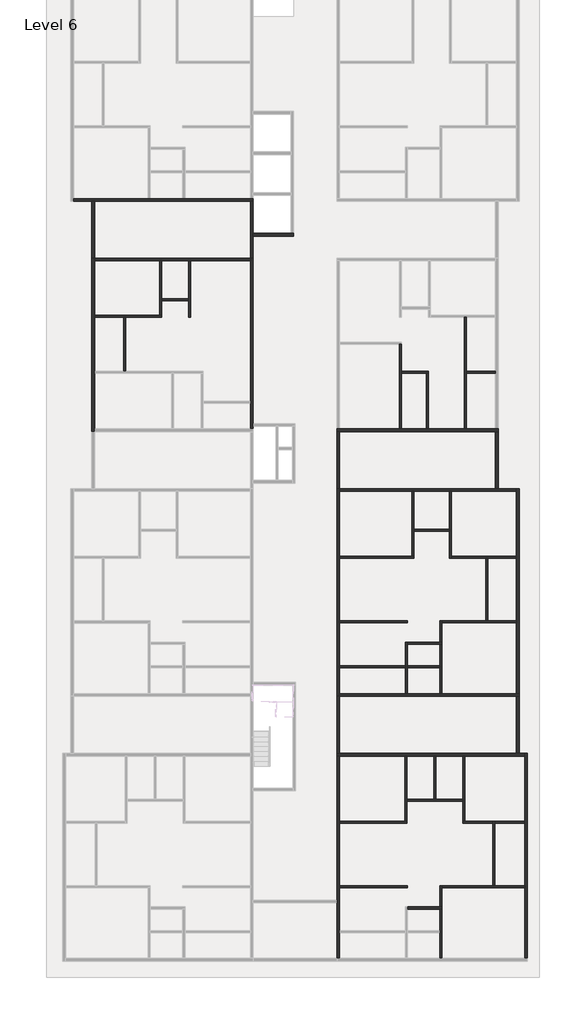
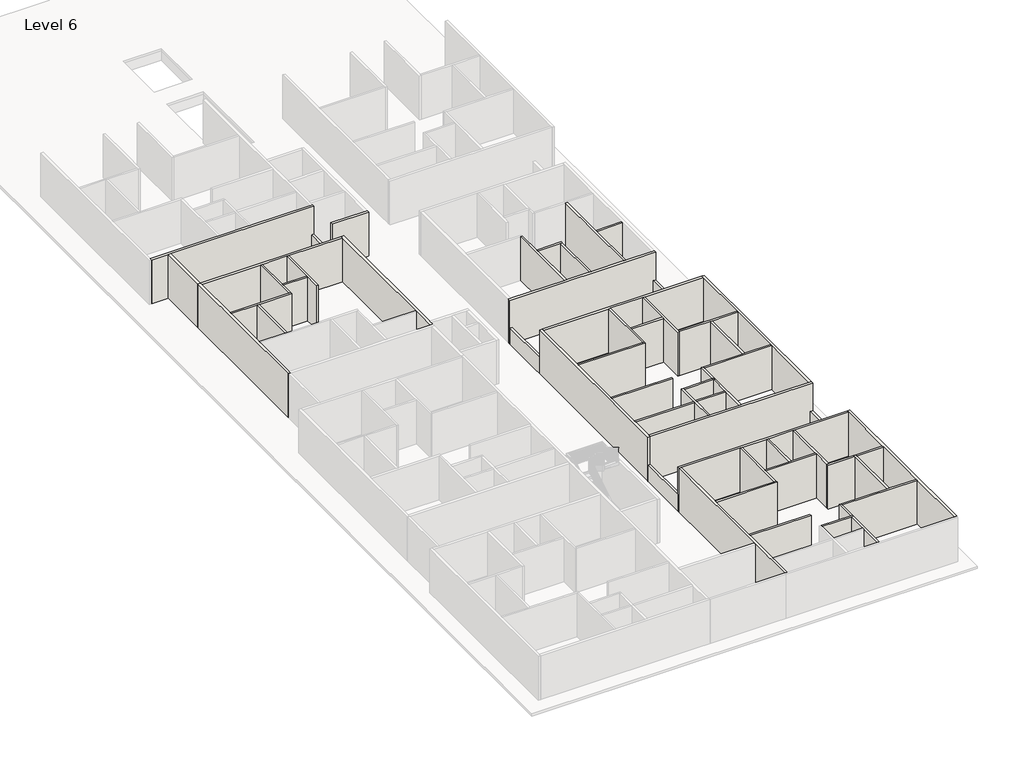
# One storey, part 2 of 8: 56 walls.
"""IFC4 building model written with IfcOpenShell, lengths in millimetres."""

from ifc_helpers import new_model, si_unit, frame, origin, place, context, project, spatial, polyline, outline, extrude, faceted_brep, element, save

model = new_model("IFC4")

# Units and contexts
model_context = context("Model", 3, world=origin())
ifc_project = project(units=[si_unit("LENGTHUNIT", "METRE", prefix="MILLI")], contexts=[model_context])

# Site, building, storey
site = spatial("IfcSite", under=ifc_project)
building = spatial("IfcBuilding", under=site)
storey = spatial("IfcBuildingStorey", under=building, Name="Level 6", Elevation=40474.6172466)

# Walls
placement = place(None, origin())
element("IfcWall", 1, ObjectType="4.5\"", at=placement, inside=storey, context=model_context, shape_type="Brep", body=[
    faceted_brep([(-12531.5544854, 2100.0216096, 40474.6172466), (-10907.2415084, 2100.0216096, 40474.6172466), (-10792.9415084, 2100.0216096, 40474.6172466), (-8759.6544854, 2100.0216096, 40474.6172466), (-8759.6544854, 2100.0216096, 43522.6172466), (-10792.9415084, 2100.0216096, 43522.6172466), (-10907.2415084, 2100.0216096, 43522.6172466), (-12531.5544854, 2100.0216096, 43522.6172466), (-12531.5544854, 2214.3216096, 40474.6172466), (-12531.5544854, 2214.3216096, 43522.6172466), (-8873.9544854, 2214.3216096, 43522.6172466), (-8759.6544854, 2214.3216096, 43522.6172466), (-8759.6544854, 2214.3216096, 40474.6172466), (-8873.9544854, 2214.3216096, 40474.6172466)], [[[0, 1, 2, 3, 4, 5, 6, 7]], [[8, 9, 10, 11, 12, 13]], [[3, 2, 1, 0, 8, 13, 12]], [[0, 7, 9, 8]], [[4, 3, 12, 11]], [[7, 6, 5, 4, 11, 10, 9]]]),
])
element("IfcWall", 2, ObjectType="4.5\"", at=placement, inside=storey, context=model_context, shape_type="Brep", body=[
    faceted_brep([(-8759.6544854, 2214.3216096, 40474.6172466), (-8759.6544854, 3014.4216096, 40474.6172466), (-8759.6544854, 3128.7216096, 40474.6172466), (-8759.6544854, 5264.2743917, 40474.6172466), (-8759.6544854, 5264.2743917, 43522.6172466), (-8759.6544854, 3128.7216096, 43522.6172466), (-8759.6544854, 3014.4216096, 43522.6172466), (-8759.6544854, 2214.3216096, 43522.6172466), (-8873.9544854, 2214.3216096, 40474.6172466), (-8873.9544854, 2214.3216096, 43522.6172466), (-8873.9544854, 5264.2743917, 43522.6172466), (-8873.9544854, 5264.2743917, 40474.6172466)], [[[0, 1, 2, 3, 4, 5, 6, 7]], [[8, 9, 10, 11]], [[3, 2, 1, 0, 8, 11]], [[0, 7, 9, 8]], [[4, 3, 11, 10]], [[7, 6, 5, 4, 10, 9]]]),
])
element("IfcWall", 3, ObjectType="4.5\"", at=placement, inside=storey, context=model_context, shape_type="Brep", body=[
    faceted_brep([(-7235.6544854, 5264.2743917, 40474.6172466), (-7235.6544854, 3128.7216096, 40474.6172466), (-7235.6544854, 3014.4216096, 40474.6172466), (-7235.6544854, 2100.0216096, 40474.6172466), (-7235.6544854, 2100.0216096, 43522.6172466), (-7235.6544854, 3014.4216096, 43522.6172466), (-7235.6544854, 3128.7216096, 43522.6172466), (-7235.6544854, 5264.2743917, 43522.6172466), (-7121.3544854, 5264.2743917, 40474.6172466), (-7121.3544854, 5264.2743917, 43522.6172466), (-7121.3544854, 2100.0216096, 43522.6172466), (-7121.3544854, 2100.0216096, 40474.6172466)], [[[0, 1, 2, 3, 4, 5, 6, 7]], [[8, 9, 10, 11]], [[3, 2, 1, 0, 8, 11]], [[4, 3, 11, 10]], [[0, 7, 9, 8]], [[7, 6, 5, 4, 10, 9]]]),
])
element("IfcWall", 4, ObjectType="4.5\"", at=placement, inside=storey, context=model_context, shape_type="SweptSolid", body=[
    extrude(outline(polyline([(-7235.6544854, 3014.4216096), (-8759.6544854, 3014.4216096), (-8759.6544854, 3128.7216096), (-7235.6544854, 3128.7216096), (-7235.6544854, 3014.4216096)])), frame((0.0, 0.0, 40474.6172466), z_axis=(0.0, 0.0, 1.0), x_axis=(1.0, 0.0, 0.0)), (0.0, 0.0, 1.0), 3048.0),
])
element("IfcWall", 5, ObjectType="4.5\"", at=placement, inside=storey, context=model_context, shape_type="SweptSolid", body=[
    extrude(outline(polyline([(-10907.2415084, -947.4344126), (-10907.2415084, 2100.0216096), (-10792.9415084, 2100.0216096), (-10792.9415084, -947.4344126), (-10907.2415084, -947.4344126)])), frame((0.0, 0.0, 40474.6172466), z_axis=(0.0, 0.0, 1.0), x_axis=(1.0, 0.0, 0.0)), (0.0, 0.0, 1.0), 3048.0),
])
element("IfcWall", 6, ObjectType="4.5\"", at=placement, inside=storey, context=model_context, shape_type="Brep", body=[
    faceted_brep([(5056.6584916, -31173.4344126, 40474.6172466), (6885.4584916, -31173.4344126, 40474.6172466), (6999.7584916, -31173.4344126, 40474.6172466), (6999.7584916, -31173.4344126, 43522.6172466), (6885.4584916, -31173.4344126, 43522.6172466), (5056.6584916, -31173.4344126, 43522.6172466), (5056.6584916, -31059.1344126, 40474.6172466), (5056.6584916, -31059.1344126, 43522.6172466), (6885.4584916, -31059.1344126, 43522.6172466), (6999.7584916, -31059.1344126, 43522.6172466), (6999.7584916, -31059.1344126, 40474.6172466), (6885.4584916, -31059.1344126, 40474.6172466)], [[[0, 1, 2, 3, 4, 5]], [[6, 7, 8, 9, 10, 11]], [[2, 1, 0, 6, 11, 10]], [[0, 5, 7, 6]], [[3, 2, 10, 9]], [[5, 4, 3, 9, 8, 7]]]),
])
element("IfcWall", 7, ObjectType="4.5\"", at=placement, inside=storey, context=model_context, shape_type="Brep", body=[
    faceted_brep([(6885.4584916, -31173.4344126, 40474.6172466), (6885.4584916, -32392.6344126, 40474.6172466), (6885.4584916, -32506.9344126, 40474.6172466), (6885.4584916, -33954.7344126, 40474.6172466), (6885.4584916, -33954.7344126, 43522.6172466), (6885.4584916, -32506.9344126, 43522.6172466), (6885.4584916, -32392.6344126, 43522.6172466), (6885.4584916, -31173.4344126, 43522.6172466), (6999.7584916, -31173.4344126, 40474.6172466), (6999.7584916, -31173.4344126, 43522.6172466), (6999.7584916, -33954.7344126, 43522.6172466), (6999.7584916, -33954.7344126, 40474.6172466)], [[[0, 1, 2, 3, 4, 5, 6, 7]], [[8, 9, 10, 11]], [[3, 2, 1, 0, 8, 11]], [[0, 7, 9, 8]], [[4, 3, 11, 10]], [[7, 6, 5, 4, 10, 9]]]),
])
element("IfcWall", 8, ObjectType="4.5\"", at=placement, inside=storey, context=model_context, shape_type="Brep", body=[
    faceted_brep([(6999.7584916, -31059.1344126, 40474.6172466), (6999.7584916, -29966.9344126, 40474.6172466), (6999.7584916, -29852.6344126, 40474.6172466), (6999.7584916, -29852.6344126, 43522.6172466), (6999.7584916, -29966.9344126, 43522.6172466), (6999.7584916, -31059.1344126, 43522.6172466), (6885.4584916, -31059.1344126, 40474.6172466), (6885.4584916, -31059.1344126, 43522.6172466), (6885.4584916, -29852.6344126, 43522.6172466), (6885.4584916, -29852.6344126, 40474.6172466)], [[[0, 1, 2, 3, 4, 5]], [[6, 7, 8, 9]], [[2, 1, 0, 6, 9]], [[0, 5, 7, 6]], [[3, 2, 9, 8]], [[5, 4, 3, 8, 7]]]),
])
element("IfcWall", 9, ObjectType="4.5\"", at=placement, inside=storey, context=model_context, shape_type="Brep", body=[
    faceted_brep([(6999.7584916, -29966.9344126, 40474.6172466), (11660.6584916, -29966.9344126, 40474.6172466), (11660.6584916, -29966.9344126, 43522.6172466), (6999.7584916, -29966.9344126, 43522.6172466), (6999.7584916, -29852.6344126, 40474.6172466), (6999.7584916, -29852.6344126, 43522.6172466), (9869.9584916, -29852.6344126, 43522.6172466), (9984.2584916, -29852.6344126, 43522.6172466), (11660.6584916, -29852.6344126, 43522.6172466), (11660.6584916, -29852.6344126, 40474.6172466), (9984.2584916, -29852.6344126, 40474.6172466), (9869.9584916, -29852.6344126, 40474.6172466)], [[[0, 1, 2, 3]], [[4, 5, 6, 7, 8, 9, 10, 11]], [[1, 0, 4, 11, 10, 9]], [[0, 3, 5, 4]], [[2, 1, 9, 8]], [[3, 2, 8, 7, 6, 5]]]),
])
element("IfcWall", 10, ObjectType="4.5\"", at=placement, inside=storey, context=model_context, shape_type="SweptSolid", body=[
    extrude(outline(polyline([(5056.6584916, -29966.9344126), (1259.3584916, -29966.9344126), (1259.3584916, -29852.6344126), (5056.6584916, -29852.6344126), (5056.6584916, -29966.9344126)])), frame((0.0, 0.0, 40474.6172466), z_axis=(0.0, 0.0, 1.0), x_axis=(1.0, 0.0, 0.0)), (0.0, 0.0, 1.0), 3048.0),
])
element("IfcWall", 11, ObjectType="4.5\"", at=placement, inside=storey, context=model_context, shape_type="Brep", body=[
    faceted_brep([(1259.3584916, -26347.4344126, 40474.6172466), (5031.2584916, -26347.4344126, 40474.6172466), (5031.2584916, -26347.4344126, 43522.6172466), (1259.3584916, -26347.4344126, 43522.6172466), (1259.3584916, -26233.1344126, 40474.6172466), (1259.3584916, -26233.1344126, 43522.6172466), (4916.9584916, -26233.1344126, 43522.6172466), (5031.2584916, -26233.1344126, 43522.6172466), (5031.2584916, -26233.1344126, 40474.6172466), (4916.9584916, -26233.1344126, 40474.6172466)], [[[0, 1, 2, 3]], [[4, 5, 6, 7, 8, 9]], [[1, 0, 4, 9, 8]], [[0, 3, 5, 4]], [[2, 1, 8, 7]], [[3, 2, 7, 6, 5]]]),
])
element("IfcWall", 12, ObjectType="4.5\"", at=placement, inside=storey, context=model_context, shape_type="Brep", body=[
    faceted_brep([(5031.2584916, -26233.1344126, 40474.6172466), (5031.2584916, -25128.2344126, 40474.6172466), (5031.2584916, -25013.9344126, 40474.6172466), (5031.2584916, -22575.5344126, 40474.6172466), (5031.2584916, -22575.5344126, 43522.6172466), (5031.2584916, -25013.9344126, 43522.6172466), (5031.2584916, -25128.2344126, 43522.6172466), (5031.2584916, -26233.1344126, 43522.6172466), (4916.9584916, -26233.1344126, 40474.6172466), (4916.9584916, -26233.1344126, 43522.6172466), (4916.9584916, -22575.5344126, 43522.6172466), (4916.9584916, -22575.5344126, 40474.6172466)], [[[0, 1, 2, 3, 4, 5, 6, 7]], [[8, 9, 10, 11]], [[3, 2, 1, 0, 8, 11]], [[0, 7, 9, 8]], [[4, 3, 11, 10]], [[7, 6, 5, 4, 10, 9]]]),
])
element("IfcWall", 13, ObjectType="4.5\"", at=placement, inside=storey, context=model_context, shape_type="Brep", body=[
    faceted_brep([(9984.2584916, -29852.6344126, 40474.6172466), (9984.2584916, -26347.4344126, 40474.6172466), (9984.2584916, -26233.1344126, 40474.6172466), (9984.2584916, -26233.1344126, 43522.6172466), (9984.2584916, -26347.4344126, 43522.6172466), (9984.2584916, -29852.6344126, 43522.6172466), (9869.9584916, -29852.6344126, 40474.6172466), (9869.9584916, -29852.6344126, 43522.6172466), (9869.9584916, -26347.4344126, 43522.6172466), (9869.9584916, -26233.1344126, 43522.6172466), (9869.9584916, -26233.1344126, 40474.6172466), (9869.9584916, -26347.4344126, 40474.6172466)], [[[0, 1, 2, 3, 4, 5]], [[6, 7, 8, 9, 10, 11]], [[2, 1, 0, 6, 11, 10]], [[0, 5, 7, 6]], [[3, 2, 10, 9]], [[5, 4, 3, 9, 8, 7]]]),
])
element("IfcWall", 14, ObjectType="4.5\"", at=placement, inside=storey, context=model_context, shape_type="SweptSolid", body=[
    extrude(outline(polyline([(11660.6584916, -26347.4344126), (9984.2584916, -26347.4344126), (9984.2584916, -26233.1344126), (11660.6584916, -26233.1344126), (11660.6584916, -26347.4344126)])), frame((0.0, 0.0, 40474.6172466), z_axis=(0.0, 0.0, 1.0), x_axis=(1.0, 0.0, 0.0)), (0.0, 0.0, 1.0), 3048.0),
])
element("IfcWall", 15, ObjectType="4.5\"", at=placement, inside=storey, context=model_context, shape_type="Brep", body=[
    faceted_brep([(9869.9584916, -26233.1344126, 40474.6172466), (8307.8584916, -26233.1344126, 40474.6172466), (8193.5584916, -26233.1344126, 40474.6172466), (8193.5584916, -26233.1344126, 43522.6172466), (8307.8584916, -26233.1344126, 43522.6172466), (9869.9584916, -26233.1344126, 43522.6172466), (9869.9584916, -26347.4344126, 40474.6172466), (9869.9584916, -26347.4344126, 43522.6172466), (8193.5584916, -26347.4344126, 43522.6172466), (8193.5584916, -26347.4344126, 40474.6172466)], [[[0, 1, 2, 3, 4, 5]], [[6, 7, 8, 9]], [[2, 1, 0, 6, 9]], [[0, 5, 7, 6]], [[3, 2, 9, 8]], [[5, 4, 3, 8, 7]]]),
])
element("IfcWall", 16, ObjectType="4.5\"", at=placement, inside=storey, context=model_context, shape_type="Brep", body=[
    faceted_brep([(8307.8584916, -26233.1344126, 40474.6172466), (8307.8584916, -22575.5344126, 40474.6172466), (8307.8584916, -22575.5344126, 43522.6172466), (8307.8584916, -26233.1344126, 43522.6172466), (8193.5584916, -26233.1344126, 40474.6172466), (8193.5584916, -26233.1344126, 43522.6172466), (8193.5584916, -25128.2344126, 43522.6172466), (8193.5584916, -25013.9344126, 43522.6172466), (8193.5584916, -22575.5344126, 43522.6172466), (8193.5584916, -22575.5344126, 40474.6172466), (8193.5584916, -25013.9344126, 40474.6172466), (8193.5584916, -25128.2344126, 40474.6172466)], [[[0, 1, 2, 3]], [[4, 5, 6, 7, 8, 9, 10, 11]], [[1, 0, 4, 11, 10, 9]], [[0, 3, 5, 4]], [[2, 1, 9, 8]], [[3, 2, 8, 7, 6, 5]]]),
])
element("IfcWall", 17, ObjectType="4.5\"", at=placement, inside=storey, context=model_context, shape_type="Brep", body=[
    faceted_brep([(5031.2584916, -25128.2344126, 40474.6172466), (8193.5584916, -25128.2344126, 40474.6172466), (8193.5584916, -25128.2344126, 43522.6172466), (5031.2584916, -25128.2344126, 43522.6172466), (5031.2584916, -25013.9344126, 40474.6172466), (5031.2584916, -25013.9344126, 43522.6172466), (6555.2584916, -25013.9344126, 43522.6172466), (6669.5584916, -25013.9344126, 43522.6172466), (8193.5584916, -25013.9344126, 43522.6172466), (8193.5584916, -25013.9344126, 40474.6172466), (6669.5584916, -25013.9344126, 40474.6172466), (6555.2584916, -25013.9344126, 40474.6172466)], [[[0, 1, 2, 3]], [[4, 5, 6, 7, 8, 9, 10, 11]], [[1, 0, 4, 11, 10, 9]], [[0, 3, 5, 4]], [[2, 1, 9, 8]], [[3, 2, 8, 7, 6, 5]]]),
])
element("IfcWall", 18, ObjectType="4.5\"", at=placement, inside=storey, context=model_context, shape_type="SweptSolid", body=[
    extrude(outline(polyline([(6555.2584916, -25013.9344126), (6555.2584916, -22575.5344126), (6669.5584916, -22575.5344126), (6669.5584916, -25013.9344126), (6555.2584916, -25013.9344126)])), frame((0.0, 0.0, 40474.6172466), z_axis=(0.0, 0.0, 1.0), x_axis=(1.0, 0.0, 0.0)), (0.0, 0.0, 1.0), 3048.0),
])
element("IfcWall", 19, ObjectType="4.5\"", at=placement, inside=storey, context=model_context, shape_type="SweptSolid", body=[
    extrude(outline(polyline([(4942.3584916, -17622.5344126), (1259.3584916, -17622.5344126), (1259.3584916, -17508.2344126), (4942.3584916, -17508.2344126), (4942.3584916, -17622.5344126)])), frame((0.0, 0.0, 40474.6172466), z_axis=(0.0, 0.0, 1.0), x_axis=(1.0, 0.0, 0.0)), (0.0, 0.0, 1.0), 3048.0),
])
element("IfcWall", 20, ObjectType="4.5\"", at=placement, inside=storey, context=model_context, shape_type="Brep", body=[
    faceted_brep([(4942.3584916, -16174.7344126, 40474.6172466), (4942.3584916, -17508.2344126, 40474.6172466), (4942.3584916, -17622.5344126, 40474.6172466), (4942.3584916, -19070.3344126, 40474.6172466), (4942.3584916, -19070.3344126, 43522.6172466), (4942.3584916, -17622.5344126, 43522.6172466), (4942.3584916, -17508.2344126, 43522.6172466), (4942.3584916, -16174.7344126, 43522.6172466), (5056.6584916, -16174.7344126, 40474.6172466), (5056.6584916, -16174.7344126, 43522.6172466), (5056.6584916, -16289.0344126, 43522.6172466), (5056.6584916, -17508.2344126, 43522.6172466), (5056.6584916, -17622.5344126, 43522.6172466), (5056.6584916, -19070.3344126, 43522.6172466), (5056.6584916, -19070.3344126, 40474.6172466), (5056.6584916, -17622.5344126, 40474.6172466), (5056.6584916, -17508.2344126, 40474.6172466), (5056.6584916, -16289.0344126, 40474.6172466)], [[[0, 1, 2, 3, 4, 5, 6, 7]], [[8, 9, 10, 11, 12, 13, 14, 15, 16, 17]], [[3, 2, 1, 0, 8, 17, 16, 15, 14]], [[4, 3, 14, 13]], [[0, 7, 9, 8]], [[7, 6, 5, 4, 13, 12, 11, 10, 9]]]),
])
element("IfcWall", 21, ObjectType="4.5\"", at=placement, inside=storey, context=model_context, shape_type="Brep", body=[
    faceted_brep([(5056.6584916, -16289.0344126, 40474.6172466), (6885.4584916, -16289.0344126, 40474.6172466), (6999.7584916, -16289.0344126, 40474.6172466), (6999.7584916, -16289.0344126, 43522.6172466), (6885.4584916, -16289.0344126, 43522.6172466), (5056.6584916, -16289.0344126, 43522.6172466), (5056.6584916, -16174.7344126, 40474.6172466), (5056.6584916, -16174.7344126, 43522.6172466), (6885.4584916, -16174.7344126, 43522.6172466), (6999.7584916, -16174.7344126, 43522.6172466), (6999.7584916, -16174.7344126, 40474.6172466), (6885.4584916, -16174.7344126, 40474.6172466)], [[[0, 1, 2, 3, 4, 5]], [[6, 7, 8, 9, 10, 11]], [[2, 1, 0, 6, 11, 10]], [[0, 5, 7, 6]], [[3, 2, 10, 9]], [[5, 4, 3, 9, 8, 7]]]),
])
element("IfcWall", 22, ObjectType="4.5\"", at=placement, inside=storey, context=model_context, shape_type="Brep", body=[
    faceted_brep([(6885.4584916, -16289.0344126, 40474.6172466), (6885.4584916, -17508.2344126, 40474.6172466), (6885.4584916, -17622.5344126, 40474.6172466), (6885.4584916, -19070.3344126, 40474.6172466), (6885.4584916, -19070.3344126, 43522.6172466), (6885.4584916, -17622.5344126, 43522.6172466), (6885.4584916, -17508.2344126, 43522.6172466), (6885.4584916, -16289.0344126, 43522.6172466), (6999.7584916, -16289.0344126, 40474.6172466), (6999.7584916, -16289.0344126, 43522.6172466), (6999.7584916, -19070.3344126, 43522.6172466), (6999.7584916, -19070.3344126, 40474.6172466)], [[[0, 1, 2, 3, 4, 5, 6, 7]], [[8, 9, 10, 11]], [[3, 2, 1, 0, 8, 11]], [[0, 7, 9, 8]], [[4, 3, 11, 10]], [[7, 6, 5, 4, 10, 9]]]),
])
element("IfcWall", 23, ObjectType="4.5\"", at=placement, inside=storey, context=model_context, shape_type="SweptSolid", body=[
    extrude(outline(polyline([(6885.4584916, -17622.5344126), (5056.6584916, -17622.5344126), (5056.6584916, -17508.2344126), (6885.4584916, -17508.2344126), (6885.4584916, -17622.5344126)])), frame((0.0, 0.0, 40474.6172466), z_axis=(0.0, 0.0, 1.0), x_axis=(1.0, 0.0, 0.0)), (0.0, 0.0, 1.0), 3048.0),
])
element("IfcWall", 24, ObjectType="4.5\"", at=placement, inside=storey, context=model_context, shape_type="Brep", body=[
    faceted_brep([(6999.7584916, -16174.7344126, 40474.6172466), (6999.7584916, -15082.5344126, 40474.6172466), (6999.7584916, -14968.2344126, 40474.6172466), (6999.7584916, -14968.2344126, 43522.6172466), (6999.7584916, -15082.5344126, 43522.6172466), (6999.7584916, -16174.7344126, 43522.6172466), (6885.4584916, -16174.7344126, 40474.6172466), (6885.4584916, -16174.7344126, 43522.6172466), (6885.4584916, -14968.2344126, 43522.6172466), (6885.4584916, -14968.2344126, 40474.6172466)], [[[0, 1, 2, 3, 4, 5]], [[6, 7, 8, 9]], [[2, 1, 0, 6, 9]], [[0, 5, 7, 6]], [[3, 2, 9, 8]], [[5, 4, 3, 8, 7]]]),
])
element("IfcWall", 25, ObjectType="4.5\"", at=placement, inside=storey, context=model_context, shape_type="Brep", body=[
    faceted_brep([(6999.7584916, -15082.5344126, 40474.6172466), (11208.5214687, -15082.5344126, 40474.6172466), (11208.5214687, -15082.5344126, 43522.6172466), (6999.7584916, -15082.5344126, 43522.6172466), (6999.7584916, -14968.2344126, 40474.6172466), (6999.7584916, -14968.2344126, 43522.6172466), (9469.9084916, -14968.2344126, 43522.6172466), (9584.2084916, -14968.2344126, 43522.6172466), (11208.5214687, -14968.2344126, 43522.6172466), (11208.5214687, -14968.2344126, 40474.6172466), (9584.2084916, -14968.2344126, 40474.6172466), (9469.9084916, -14968.2344126, 40474.6172466)], [[[0, 1, 2, 3]], [[4, 5, 6, 7, 8, 9, 10, 11]], [[1, 0, 4, 11, 10, 9]], [[0, 3, 5, 4]], [[2, 1, 9, 8]], [[3, 2, 8, 7, 6, 5]]]),
])
element("IfcWall", 26, ObjectType="4.5\"", at=placement, inside=storey, context=model_context, shape_type="SweptSolid", body=[
    extrude(outline(polyline([(5056.6584916, -15082.5344126), (1259.3584916, -15082.5344126), (1259.3584916, -14968.2344126), (5056.6584916, -14968.2344126), (5056.6584916, -15082.5344126)])), frame((0.0, 0.0, 40474.6172466), z_axis=(0.0, 0.0, 1.0), x_axis=(1.0, 0.0, 0.0)), (0.0, 0.0, 1.0), 3048.0),
])
element("IfcWall", 27, ObjectType="4.5\"", at=placement, inside=storey, context=model_context, shape_type="Brep", body=[
    faceted_brep([(1259.3584916, -11463.0344126, 40474.6172466), (5430.0214687, -11463.0344126, 40474.6172466), (5430.0214687, -11463.0344126, 43522.6172466), (1259.3584916, -11463.0344126, 43522.6172466), (1259.3584916, -11348.7344126, 40474.6172466), (1259.3584916, -11348.7344126, 43522.6172466), (5315.7214687, -11348.7344126, 43522.6172466), (5430.0214687, -11348.7344126, 43522.6172466), (5430.0214687, -11348.7344126, 40474.6172466), (5315.7214687, -11348.7344126, 40474.6172466)], [[[0, 1, 2, 3]], [[4, 5, 6, 7, 8, 9]], [[1, 0, 4, 9, 8]], [[0, 3, 5, 4]], [[2, 1, 8, 7]], [[3, 2, 7, 6, 5]]]),
])
element("IfcWall", 28, ObjectType="4.5\"", at=placement, inside=storey, context=model_context, shape_type="Brep", body=[
    faceted_brep([(5430.0214687, -11348.7344126, 40474.6172466), (5430.0214687, -9939.0344126, 40474.6172466), (5430.0214687, -9824.7344126, 40474.6172466), (5430.0214687, -7691.1344126, 40474.6172466), (5430.0214687, -7691.1344126, 43522.6172466), (5430.0214687, -9824.7344126, 43522.6172466), (5430.0214687, -9939.0344126, 43522.6172466), (5430.0214687, -11348.7344126, 43522.6172466), (5315.7214687, -11348.7344126, 40474.6172466), (5315.7214687, -11348.7344126, 43522.6172466), (5315.7214687, -7691.1344126, 43522.6172466), (5315.7214687, -7691.1344126, 40474.6172466)], [[[0, 1, 2, 3, 4, 5, 6, 7]], [[8, 9, 10, 11]], [[3, 2, 1, 0, 8, 11]], [[0, 7, 9, 8]], [[4, 3, 11, 10]], [[7, 6, 5, 4, 10, 9]]]),
])
element("IfcWall", 29, ObjectType="4.5\"", at=placement, inside=storey, context=model_context, shape_type="SweptSolid", body=[
    extrude(outline(polyline([(7436.6214687, -9939.0344126), (5430.0214687, -9939.0344126), (5430.0214687, -9824.7344126), (7436.6214687, -9824.7344126), (7436.6214687, -9939.0344126)])), frame((0.0, 0.0, 40474.6172466), z_axis=(0.0, 0.0, 1.0), x_axis=(1.0, 0.0, 0.0)), (0.0, 0.0, 1.0), 3048.0),
])
element("IfcWall", 30, ObjectType="4.5\"", at=placement, inside=storey, context=model_context, shape_type="Brep", body=[
    faceted_brep([(7436.6214687, -7691.1344126, 40474.6172466), (7436.6214687, -9824.7344126, 40474.6172466), (7436.6214687, -9939.0344126, 40474.6172466), (7436.6214687, -11463.0344126, 40474.6172466), (7436.6214687, -11463.0344126, 43522.6172466), (7436.6214687, -9939.0344126, 43522.6172466), (7436.6214687, -9824.7344126, 43522.6172466), (7436.6214687, -7691.1344126, 43522.6172466), (7550.9214687, -7691.1344126, 40474.6172466), (7550.9214687, -7691.1344126, 43522.6172466), (7550.9214687, -11348.7344126, 43522.6172466), (7550.9214687, -11463.0344126, 43522.6172466), (7550.9214687, -11463.0344126, 40474.6172466), (7550.9214687, -11348.7344126, 40474.6172466)], [[[0, 1, 2, 3, 4, 5, 6, 7]], [[8, 9, 10, 11, 12, 13]], [[3, 2, 1, 0, 8, 13, 12]], [[0, 7, 9, 8]], [[4, 3, 12, 11]], [[7, 6, 5, 4, 11, 10, 9]]]),
])
element("IfcWall", 31, ObjectType="4.5\"", at=placement, inside=storey, context=model_context, shape_type="Brep", body=[
    faceted_brep([(7550.9214687, -11463.0344126, 40474.6172466), (9469.9084916, -11463.0344126, 40474.6172466), (9584.2084916, -11463.0344126, 40474.6172466), (11208.5214687, -11463.0344126, 40474.6172466), (11208.5214687, -11463.0344126, 43522.6172466), (9584.2084916, -11463.0344126, 43522.6172466), (9469.9084916, -11463.0344126, 43522.6172466), (7550.9214687, -11463.0344126, 43522.6172466), (7550.9214687, -11348.7344126, 40474.6172466), (7550.9214687, -11348.7344126, 43522.6172466), (11208.5214687, -11348.7344126, 43522.6172466), (11208.5214687, -11348.7344126, 40474.6172466)], [[[0, 1, 2, 3, 4, 5, 6, 7]], [[8, 9, 10, 11]], [[3, 2, 1, 0, 8, 11]], [[0, 7, 9, 8]], [[4, 3, 11, 10]], [[7, 6, 5, 4, 10, 9]]]),
])
element("IfcWall", 32, ObjectType="4.5\"", at=placement, inside=storey, context=model_context, shape_type="SweptSolid", body=[
    extrude(outline(polyline([(9469.9084916, -14968.2344126), (9469.9084916, -11463.0344126), (9584.2084916, -11463.0344126), (9584.2084916, -14968.2344126), (9469.9084916, -14968.2344126)])), frame((0.0, 0.0, 40474.6172466), z_axis=(0.0, 0.0, 1.0), x_axis=(1.0, 0.0, 0.0)), (0.0, 0.0, 1.0), 3048.0),
])
element("IfcWall", 33, ObjectType="4.5\"", at=placement, inside=storey, context=model_context, shape_type="Brep", body=[
    faceted_brep([(4610.8714687, 572.7745083, 40474.6172466), (4610.8714687, -4185.9344126, 40474.6172466), (4610.8714687, -4185.9344126, 43522.6172466), (4610.8714687, 572.7745083, 43522.6172466), (4725.1714687, 572.7745083, 40474.6172466), (4725.1714687, 572.7745083, 43522.6172466), (4725.1714687, -947.4344126, 43522.6172466), (4725.1714687, -1061.7344126, 43522.6172466), (4725.1714687, -4185.9344126, 43522.6172466), (4725.1714687, -4185.9344126, 40474.6172466), (4725.1714687, -1061.7344126, 40474.6172466), (4725.1714687, -947.4344126, 40474.6172466)], [[[0, 1, 2, 3]], [[4, 5, 6, 7, 8, 9, 10, 11]], [[1, 0, 4, 11, 10, 9]], [[0, 3, 5, 4]], [[2, 1, 9, 8]], [[3, 2, 8, 7, 6, 5]]]),
])
element("IfcWall", 34, ObjectType="4.5\"", at=placement, inside=storey, context=model_context, shape_type="Brep", body=[
    faceted_brep([(4725.1714687, -1061.7344126, 40474.6172466), (6134.8714687, -1061.7344126, 40474.6172466), (6249.1714687, -1061.7344126, 40474.6172466), (6249.1714687, -1061.7344126, 43522.6172466), (6134.8714687, -1061.7344126, 43522.6172466), (4725.1714687, -1061.7344126, 43522.6172466), (4725.1714687, -947.4344126, 40474.6172466), (4725.1714687, -947.4344126, 43522.6172466), (6249.1714687, -947.4344126, 43522.6172466), (6249.1714687, -947.4344126, 40474.6172466)], [[[0, 1, 2, 3, 4, 5]], [[6, 7, 8, 9]], [[2, 1, 0, 6, 9]], [[0, 5, 7, 6]], [[3, 2, 9, 8]], [[5, 4, 3, 8, 7]]]),
])
element("IfcWall", 35, ObjectType="4.5\"", at=placement, inside=storey, context=model_context, shape_type="SweptSolid", body=[
    extrude(outline(polyline([(6134.8714687, -4185.9344126), (6134.8714687, -1061.7344126), (6249.1714687, -1061.7344126), (6249.1714687, -4185.9344126), (6134.8714687, -4185.9344126)])), frame((0.0, 0.0, 40474.6172466), z_axis=(0.0, 0.0, 1.0), x_axis=(1.0, 0.0, 0.0)), (0.0, 0.0, 1.0), 3048.0),
])
element("IfcWall", 36, ObjectType="4.5\"", at=placement, inside=storey, context=model_context, shape_type="Brep", body=[
    faceted_brep([(8396.7584916, -4185.9344126, 40474.6172466), (8396.7584916, -1061.7344126, 40474.6172466), (8396.7584916, -947.4344126, 40474.6172466), (8396.7584916, 2100.0216096, 40474.6172466), (8396.7584916, 2100.0216096, 43522.6172466), (8396.7584916, -947.4344126, 43522.6172466), (8396.7584916, -1061.7344126, 43522.6172466), (8396.7584916, -4185.9344126, 43522.6172466), (8282.4584916, -4185.9344126, 40474.6172466), (8282.4584916, -4185.9344126, 43522.6172466), (8282.4584916, 2100.0216096, 43522.6172466), (8282.4584916, 2100.0216096, 40474.6172466)], [[[0, 1, 2, 3, 4, 5, 6, 7]], [[8, 9, 10, 11]], [[3, 2, 1, 0, 8, 11]], [[0, 7, 9, 8]], [[4, 3, 11, 10]], [[7, 6, 5, 4, 10, 9]]]),
])
element("IfcWall", 37, ObjectType="4.5\"", at=placement, inside=storey, context=model_context, shape_type="SweptSolid", body=[
    extrude(outline(polyline([(8396.7584916, -947.4344126), (10021.0714687, -947.4344126), (10021.0714687, -1061.7344126), (8396.7584916, -1061.7344126), (8396.7584916, -947.4344126)])), frame((0.0, 0.0, 40474.6172466), z_axis=(0.0, 0.0, 1.0), x_axis=(1.0, 0.0, 0.0)), (0.0, 0.0, 1.0), 3048.0),
])
element("IfcWall", 38, ObjectType="6\"", at=placement, inside=storey, context=model_context, shape_type="Brep", body=[
    faceted_brep([(-13719.0044854, 8615.1216096, 40474.6172466), (-12683.9544854, 8615.1216096, 40474.6172466), (-12531.5544854, 8615.1216096, 40474.6172466), (-3769.8415084, 8615.1216096, 40474.6172466), (-3617.4415084, 8615.1216096, 40474.6172466), (-3617.4415084, 8615.1216096, 41693.8172466), (-3617.4415084, 8615.1216096, 43522.6172466), (-12531.5544854, 8615.1216096, 43522.6172466), (-12683.9544854, 8615.1216096, 43522.6172466), (-13719.0044854, 8615.1216096, 43522.6172466), (-13719.0044854, 8767.5216096, 40474.6172466), (-13719.0044854, 8767.5216096, 43522.6172466), (-9510.2415084, 8767.5216096, 43522.6172466), (-9395.9415084, 8767.5216096, 43522.6172466), (-7567.1415084, 8767.5216096, 43522.6172466), (-7452.8415084, 8767.5216096, 43522.6172466), (-3769.8415084, 8767.5216096, 43522.6172466), (-3617.4415084, 8767.5216096, 43522.6172466), (-3617.4415084, 8767.5216096, 40474.6172466), (-3769.8415084, 8767.5216096, 40474.6172466), (-7452.8415084, 8767.5216096, 40474.6172466), (-7567.1415084, 8767.5216096, 40474.6172466), (-9395.9415084, 8767.5216096, 40474.6172466), (-9510.2415084, 8767.5216096, 40474.6172466)], [[[0, 1, 2, 3, 4, 5, 6, 7, 8, 9]], [[10, 11, 12, 13, 14, 15, 16, 17, 18, 19, 20, 21, 22, 23]], [[4, 3, 2, 1, 0, 10, 23, 22, 21, 20, 19, 18]], [[0, 9, 11, 10]], [[4, 18, 17, 6, 5]], [[9, 8, 7, 6, 17, 16, 15, 14, 13, 12, 11]]]),
])
element("IfcWall", 39, ObjectType="6\"", at=placement, inside=storey, context=model_context, shape_type="Brep", body=[
    faceted_brep([(-12683.9544854, 5416.6743917, 40474.6172466), (-12683.9544854, -4338.3344126, 40474.6172466), (-12683.9544854, -4338.3344126, 43522.6172466), (-12683.9544854, 5416.6743917, 43522.6172466), (-12531.5544854, 5416.6743917, 40474.6172466), (-12531.5544854, 5416.6743917, 43522.6172466), (-12531.5544854, 5264.2743917, 43522.6172466), (-12531.5544854, 2214.3216096, 43522.6172466), (-12531.5544854, 2100.0216096, 43522.6172466), (-12531.5544854, -947.4344126, 43522.6172466), (-12531.5544854, -1061.7344126, 43522.6172466), (-12531.5544854, -4185.9344126, 43522.6172466), (-12531.5544854, -4338.3344126, 43522.6172466), (-12531.5544854, -4338.3344126, 40474.6172466), (-12531.5544854, -4185.9344126, 40474.6172466), (-12531.5544854, -1061.7344126, 40474.6172466), (-12531.5544854, -947.4344126, 40474.6172466), (-12531.5544854, 2100.0216096, 40474.6172466), (-12531.5544854, 2214.3216096, 40474.6172466), (-12531.5544854, 5264.2743917, 40474.6172466)], [[[0, 1, 2, 3]], [[4, 5, 6, 7, 8, 9, 10, 11, 12, 13, 14, 15, 16, 17, 18, 19]], [[1, 0, 4, 19, 18, 17, 16, 15, 14, 13]], [[2, 1, 13, 12]], [[0, 3, 5, 4]], [[3, 2, 12, 11, 10, 9, 8, 7, 6, 5]]]),
])
element("IfcWall", 40, ObjectType="6\"", at=placement, inside=storey, context=model_context, shape_type="Brep", body=[
    faceted_brep([(-3617.4415084, -4185.9344126, 40474.6172466), (-3617.4415084, -4034.6751812, 40474.6172466), (-3617.4415084, -3882.2751812, 40474.6172466), (-3617.4415084, 5416.6743917, 40474.6172466), (-3617.4415084, 5416.6743917, 43522.6172466), (-3617.4415084, -3882.2751812, 43522.6172466), (-3617.4415084, -4034.6751812, 43522.6172466), (-3617.4415084, -4185.9344126, 43522.6172466), (-3769.8415084, -4185.9344126, 40474.6172466), (-3769.8415084, -4185.9344126, 43522.6172466), (-3769.8415084, -2738.1344126, 43522.6172466), (-3769.8415084, -2623.8344126, 43522.6172466), (-3769.8415084, 5264.2743917, 43522.6172466), (-3769.8415084, 5416.6743917, 43522.6172466), (-3769.8415084, 5416.6743917, 40474.6172466), (-3769.8415084, 5264.2743917, 40474.6172466), (-3769.8415084, -2623.8344126, 40474.6172466), (-3769.8415084, -2738.1344126, 40474.6172466)], [[[0, 1, 2, 3, 4, 5, 6, 7]], [[8, 9, 10, 11, 12, 13, 14, 15, 16, 17]], [[3, 2, 1, 0, 8, 17, 16, 15, 14]], [[0, 7, 9, 8]], [[3, 14, 13, 4]], [[7, 6, 5, 4, 13, 12, 11, 10, 9]]]),
])
element("IfcWall", 41, ObjectType="6\"", at=placement, inside=storey, context=model_context, shape_type="Brep", body=[
    faceted_brep([(-3769.8415084, 5416.6743917, 43522.6172466), (-3769.8415084, 5416.6743917, 40474.6172466), (-12531.5544854, 5416.6743917, 40474.6172466), (-12531.5544854, 5416.6743917, 43522.6172466), (-3769.8415084, 5264.2743917, 40474.6172466), (-3769.8415084, 5264.2743917, 43522.6172466), (-7121.3544854, 5264.2743917, 43522.6172466), (-7235.6544854, 5264.2743917, 43522.6172466), (-8759.6544854, 5264.2743917, 43522.6172466), (-8873.9544854, 5264.2743917, 43522.6172466), (-12531.5544854, 5264.2743917, 43522.6172466), (-12531.5544854, 5264.2743917, 40474.6172466), (-8873.9544854, 5264.2743917, 40474.6172466), (-8759.6544854, 5264.2743917, 40474.6172466), (-7235.6544854, 5264.2743917, 40474.6172466), (-7121.3544854, 5264.2743917, 40474.6172466)], [[[0, 1, 2, 3]], [[4, 5, 6, 7, 8, 9, 10, 11, 12, 13, 14, 15]], [[2, 1, 4, 15, 14, 13, 12, 11]], [[3, 2, 11, 10]], [[0, 5, 4, 1]], [[0, 3, 10, 9, 8, 7, 6, 5]]]),
])
element("IfcWall", 42, ObjectType="6\"", at=placement, inside=storey, context=model_context, shape_type="Brep", body=[
    faceted_brep([(11813.0584916, -33954.7344126, 40474.6172466), (11813.0584916, -22423.1344126, 40474.6172466), (11813.0584916, -22423.1344126, 43522.6172466), (11813.0584916, -33954.7344126, 43522.6172466), (11660.6584916, -33954.7344126, 40474.6172466), (11660.6584916, -33954.7344126, 43522.6172466), (11660.6584916, -29966.9344126, 43522.6172466), (11660.6584916, -29852.6344126, 43522.6172466), (11660.6584916, -26347.4344126, 43522.6172466), (11660.6584916, -26233.1344126, 43522.6172466), (11660.6584916, -22575.5344126, 43522.6172466), (11660.6584916, -22423.1344126, 43522.6172466), (11660.6584916, -22423.1344126, 40474.6172466), (11660.6584916, -22575.5344126, 40474.6172466), (11660.6584916, -26233.1344126, 40474.6172466), (11660.6584916, -26347.4344126, 40474.6172466), (11660.6584916, -29852.6344126, 40474.6172466), (11660.6584916, -29966.9344126, 40474.6172466)], [[[0, 1, 2, 3]], [[4, 5, 6, 7, 8, 9, 10, 11, 12, 13, 14, 15, 16, 17]], [[1, 0, 4, 17, 16, 15, 14, 13, 12]], [[0, 3, 5, 4]], [[2, 1, 12, 11]], [[3, 2, 11, 10, 9, 8, 7, 6, 5]]]),
])
element("IfcWall", 43, ObjectType="6\"", at=placement, inside=storey, context=model_context, shape_type="Brep", body=[
    faceted_brep([(11660.6584916, -22423.1344126, 40474.6172466), (11360.9214687, -22423.1344126, 40474.6172466), (11208.5214687, -22423.1344126, 40474.6172466), (1259.3584916, -22423.1344126, 40474.6172466), (1106.9584916, -22423.1344126, 40474.6172466), (1106.9584916, -22423.1344126, 41693.8172466), (1106.9584916, -22423.1344126, 43522.6172466), (11660.6584916, -22423.1344126, 43522.6172466), (11660.6584916, -22575.5344126, 40474.6172466), (11660.6584916, -22575.5344126, 43522.6172466), (8307.8584916, -22575.5344126, 43522.6172466), (8193.5584916, -22575.5344126, 43522.6172466), (6669.5584916, -22575.5344126, 43522.6172466), (6555.2584916, -22575.5344126, 43522.6172466), (5031.2584916, -22575.5344126, 43522.6172466), (4916.9584916, -22575.5344126, 43522.6172466), (1259.3584916, -22575.5344126, 43522.6172466), (1106.9584916, -22575.5344126, 43522.6172466), (1106.9584916, -22575.5344126, 40474.6172466), (1259.3584916, -22575.5344126, 40474.6172466), (4916.9584916, -22575.5344126, 40474.6172466), (5031.2584916, -22575.5344126, 40474.6172466), (6555.2584916, -22575.5344126, 40474.6172466), (6669.5584916, -22575.5344126, 40474.6172466), (8193.5584916, -22575.5344126, 40474.6172466), (8307.8584916, -22575.5344126, 40474.6172466)], [[[0, 1, 2, 3, 4, 5, 6, 7]], [[8, 9, 10, 11, 12, 13, 14, 15, 16, 17, 18, 19, 20, 21, 22, 23, 24, 25]], [[4, 3, 2, 1, 0, 8, 25, 24, 23, 22, 21, 20, 19, 18]], [[0, 7, 9, 8]], [[4, 18, 17, 6, 5]], [[7, 6, 17, 16, 15, 14, 13, 12, 11, 10, 9]]]),
])
element("IfcWall", 44, ObjectType="6\"", at=placement, inside=storey, context=model_context, shape_type="Brep", body=[
    faceted_brep([(1106.9584916, -22575.5344126, 43522.6172466), (1106.9584916, -22575.5344126, 40474.6172466), (1106.9584916, -30668.5325185, 40474.6172466), (1106.9584916, -30820.9325185, 40474.6172466), (1106.9584916, -33954.7344126, 40474.6172466), (1106.9584916, -33954.7344126, 43522.6172466), (1106.9584916, -30820.9325185, 43522.6172466), (1106.9584916, -30668.5325185, 43522.6172466), (1259.3584916, -22575.5344126, 40474.6172466), (1259.3584916, -22575.5344126, 43522.6172466), (1259.3584916, -26233.1344126, 43522.6172466), (1259.3584916, -26347.4344126, 43522.6172466), (1259.3584916, -29852.6344126, 43522.6172466), (1259.3584916, -29966.9344126, 43522.6172466), (1259.3584916, -32392.6344126, 43522.6172466), (1259.3584916, -32506.9344126, 43522.6172466), (1259.3584916, -33954.7344126, 43522.6172466), (1259.3584916, -33954.7344126, 40474.6172466), (1259.3584916, -32506.9344126, 40474.6172466), (1259.3584916, -32392.6344126, 40474.6172466), (1259.3584916, -29966.9344126, 40474.6172466), (1259.3584916, -29852.6344126, 40474.6172466), (1259.3584916, -26347.4344126, 40474.6172466), (1259.3584916, -26233.1344126, 40474.6172466)], [[[0, 1, 2, 3, 4, 5, 6, 7]], [[8, 9, 10, 11, 12, 13, 14, 15, 16, 17, 18, 19, 20, 21, 22, 23]], [[4, 3, 2, 1, 8, 23, 22, 21, 20, 19, 18, 17]], [[5, 4, 17, 16]], [[0, 9, 8, 1]], [[0, 7, 6, 5, 16, 15, 14, 13, 12, 11, 10, 9]]]),
])
element("IfcWall", 45, ObjectType="6\"", at=placement, inside=storey, context=model_context, shape_type="Brep", body=[
    faceted_brep([(1106.9584916, -7538.7344126, 43522.6172466), (1106.9584916, -7538.7344126, 40474.6172466), (1106.9584916, -19222.7344126, 40474.6172466), (1106.9584916, -19222.7344126, 43522.6172466), (1259.3584916, -7538.7344126, 40474.6172466), (1259.3584916, -7538.7344126, 43522.6172466), (1259.3584916, -7691.1344126, 43522.6172466), (1259.3584916, -11348.7344126, 43522.6172466), (1259.3584916, -11463.0344126, 43522.6172466), (1259.3584916, -14968.2344126, 43522.6172466), (1259.3584916, -15082.5344126, 43522.6172466), (1259.3584916, -17508.2344126, 43522.6172466), (1259.3584916, -17622.5344126, 43522.6172466), (1259.3584916, -19070.3344126, 43522.6172466), (1259.3584916, -19222.7344126, 43522.6172466), (1259.3584916, -19222.7344126, 40474.6172466), (1259.3584916, -19070.3344126, 40474.6172466), (1259.3584916, -17622.5344126, 40474.6172466), (1259.3584916, -17508.2344126, 40474.6172466), (1259.3584916, -15082.5344126, 40474.6172466), (1259.3584916, -14968.2344126, 40474.6172466), (1259.3584916, -11463.0344126, 40474.6172466), (1259.3584916, -11348.7344126, 40474.6172466), (1259.3584916, -7691.1344126, 40474.6172466)], [[[0, 1, 2, 3]], [[4, 5, 6, 7, 8, 9, 10, 11, 12, 13, 14, 15, 16, 17, 18, 19, 20, 21, 22, 23]], [[2, 1, 4, 23, 22, 21, 20, 19, 18, 17, 16, 15]], [[0, 5, 4, 1]], [[2, 15, 14, 3]], [[0, 3, 14, 13, 12, 11, 10, 9, 8, 7, 6, 5]]]),
])
element("IfcWall", 46, ObjectType="6\"", at=placement, inside=storey, context=model_context, shape_type="Brep", body=[
    faceted_brep([(1259.3584916, -19222.7344126, 43522.6172466), (1259.3584916, -19222.7344126, 40474.6172466), (11208.5214687, -19222.7344126, 40474.6172466), (11360.9214687, -19222.7344126, 40474.6172466), (11360.9214687, -19222.7344126, 41693.8172466), (11360.9214687, -19222.7344126, 43522.6172466), (1259.3584916, -19070.3344126, 40474.6172466), (1259.3584916, -19070.3344126, 43522.6172466), (4942.3584916, -19070.3344126, 43522.6172466), (5056.6584916, -19070.3344126, 43522.6172466), (6885.4584916, -19070.3344126, 43522.6172466), (6999.7584916, -19070.3344126, 43522.6172466), (11208.5214687, -19070.3344126, 43522.6172466), (11360.9214687, -19070.3344126, 43522.6172466), (11360.9214687, -19070.3344126, 40474.6172466), (11208.5214687, -19070.3344126, 40474.6172466), (6999.7584916, -19070.3344126, 40474.6172466), (6885.4584916, -19070.3344126, 40474.6172466), (5056.6584916, -19070.3344126, 40474.6172466), (4942.3584916, -19070.3344126, 40474.6172466)], [[[0, 1, 2, 3, 4, 5]], [[6, 7, 8, 9, 10, 11, 12, 13, 14, 15, 16, 17, 18, 19]], [[3, 2, 1, 6, 19, 18, 17, 16, 15, 14]], [[3, 14, 13, 5, 4]], [[0, 7, 6, 1]], [[0, 5, 13, 12, 11, 10, 9, 8, 7]]]),
])
element("IfcWall", 47, ObjectType="6\"", at=placement, inside=storey, context=model_context, shape_type="Brep", body=[
    faceted_brep([(11360.9214687, -19070.3344126, 43522.6172466), (11360.9214687, -19070.3344126, 40474.6172466), (11360.9214687, -7538.7344126, 40474.6172466), (11360.9214687, -7538.7344126, 43522.6172466), (11208.5214687, -19070.3344126, 40474.6172466), (11208.5214687, -19070.3344126, 43522.6172466), (11208.5214687, -15082.5344126, 43522.6172466), (11208.5214687, -14968.2344126, 43522.6172466), (11208.5214687, -11463.0344126, 43522.6172466), (11208.5214687, -11348.7344126, 43522.6172466), (11208.5214687, -7691.1344126, 43522.6172466), (11208.5214687, -7538.7344126, 43522.6172466), (11208.5214687, -7538.7344126, 40474.6172466), (11208.5214687, -7691.1344126, 40474.6172466), (11208.5214687, -11348.7344126, 40474.6172466), (11208.5214687, -11463.0344126, 40474.6172466), (11208.5214687, -14968.2344126, 40474.6172466), (11208.5214687, -15082.5344126, 40474.6172466)], [[[0, 1, 2, 3]], [[4, 5, 6, 7, 8, 9, 10, 11, 12, 13, 14, 15, 16, 17]], [[2, 1, 4, 17, 16, 15, 14, 13, 12]], [[3, 2, 12, 11]], [[0, 5, 4, 1]], [[0, 3, 11, 10, 9, 8, 7, 6, 5]]]),
])
element("IfcWall", 48, ObjectType="6\"", at=placement, inside=storey, context=model_context, shape_type="Brep", body=[
    faceted_brep([(11208.5214687, -7538.7344126, 40474.6172466), (10173.4714687, -7538.7344126, 40474.6172466), (10021.0714687, -7538.7344126, 40474.6172466), (1259.3584916, -7538.7344126, 40474.6172466), (1259.3584916, -7538.7344126, 43522.6172466), (11208.5214687, -7538.7344126, 43522.6172466), (11208.5214687, -7691.1344126, 40474.6172466), (11208.5214687, -7691.1344126, 43522.6172466), (7550.9214687, -7691.1344126, 43522.6172466), (7436.6214687, -7691.1344126, 43522.6172466), (5430.0214687, -7691.1344126, 43522.6172466), (5315.7214687, -7691.1344126, 43522.6172466), (1259.3584916, -7691.1344126, 43522.6172466), (1259.3584916, -7691.1344126, 40474.6172466), (5315.7214687, -7691.1344126, 40474.6172466), (5430.0214687, -7691.1344126, 40474.6172466), (7436.6214687, -7691.1344126, 40474.6172466), (7550.9214687, -7691.1344126, 40474.6172466)], [[[0, 1, 2, 3, 4, 5]], [[6, 7, 8, 9, 10, 11, 12, 13, 14, 15, 16, 17]], [[3, 2, 1, 0, 6, 17, 16, 15, 14, 13]], [[0, 5, 7, 6]], [[3, 13, 12, 4]], [[5, 4, 12, 11, 10, 9, 8, 7]]]),
])
element("IfcWall", 49, ObjectType="6\"", at=placement, inside=storey, context=model_context, shape_type="Brep", body=[
    faceted_brep([(1106.9584916, -4338.3344126, 43522.6172466), (1106.9584916, -4338.3344126, 41693.8172466), (1106.9584916, -4338.3344126, 40474.6172466), (1259.3584916, -4338.3344126, 40474.6172466), (10021.0714687, -4338.3344126, 40474.6172466), (10173.4714687, -4338.3344126, 40474.6172466), (10173.4714687, -4338.3344126, 41693.8172466), (10173.4714687, -4338.3344126, 43522.6172466), (1106.9584916, -4185.9344126, 40474.6172466), (1106.9584916, -4185.9344126, 43522.6172466), (1259.3584916, -4185.9344126, 43522.6172466), (4610.8714687, -4185.9344126, 43522.6172466), (4725.1714687, -4185.9344126, 43522.6172466), (6134.8714687, -4185.9344126, 43522.6172466), (6249.1714687, -4185.9344126, 43522.6172466), (8282.4584916, -4185.9344126, 43522.6172466), (8396.7584916, -4185.9344126, 43522.6172466), (10021.0714687, -4185.9344126, 43522.6172466), (10173.4714687, -4185.9344126, 43522.6172466), (10173.4714687, -4185.9344126, 40474.6172466), (10021.0714687, -4185.9344126, 40474.6172466), (8396.7584916, -4185.9344126, 40474.6172466), (8282.4584916, -4185.9344126, 40474.6172466), (6249.1714687, -4185.9344126, 40474.6172466), (6134.8714687, -4185.9344126, 40474.6172466), (4725.1714687, -4185.9344126, 40474.6172466), (4610.8714687, -4185.9344126, 40474.6172466), (1259.3584916, -4185.9344126, 40474.6172466)], [[[0, 1, 2, 3, 4, 5, 6, 7]], [[8, 9, 10, 11, 12, 13, 14, 15, 16, 17, 18, 19, 20, 21, 22, 23, 24, 25, 26, 27]], [[5, 4, 3, 2, 8, 27, 26, 25, 24, 23, 22, 21, 20, 19]], [[0, 9, 8, 2, 1]], [[5, 19, 18, 7, 6]], [[0, 7, 18, 17, 16, 15, 14, 13, 12, 11, 10, 9]]]),
])
element("IfcWall", 50, ObjectType="6\"", at=placement, inside=storey, context=model_context, shape_type="Brep", body=[
    faceted_brep([(-3617.4415084, 6659.2303368, 40474.6172466), (-1331.4415084, 6659.2303368, 40474.6172466), (-1331.4415084, 6659.2303368, 43522.6172466), (-3617.4415084, 6659.2303368, 43522.6172466), (-3617.4415084, 6811.6303368, 40474.6172466), (-3617.4415084, 6811.6303368, 43522.6172466), (-1483.8415084, 6811.6303368, 43522.6172466), (-1331.4415084, 6811.6303368, 43522.6172466), (-1331.4415084, 6811.6303368, 40474.6172466), (-1483.8415084, 6811.6303368, 40474.6172466)], [[[0, 1, 2, 3]], [[4, 5, 6, 7, 8, 9]], [[1, 0, 4, 9, 8]], [[3, 2, 7, 6, 5]], [[0, 3, 5, 4]], [[2, 1, 8, 7]]]),
])
element("IfcWall", 51, ObjectType="6\" 2", at=placement, inside=storey, context=model_context, shape_type="SweptSolid", body=[
    extrude(outline(polyline([(-12683.9544854, 5416.6743917), (-12683.9544854, 8615.1216096), (-12531.5544854, 8615.1216096), (-12531.5544854, 5416.6743917), (-12683.9544854, 5416.6743917)])), frame((0.0, 0.0, 40474.6172466), z_axis=(0.0, 0.0, 1.0), x_axis=(1.0, 0.0, 0.0)), (0.0, 0.0, 1.0), 3048.0),
])
element("IfcWall", 52, ObjectType="6\" 2", at=placement, inside=storey, context=model_context, shape_type="Brep", body=[
    faceted_brep([(-3769.8415084, 8615.1216096, 40474.6172466), (-3769.8415084, 5416.6743917, 40474.6172466), (-3769.8415084, 5416.6743917, 41693.8172466), (-3769.8415084, 8615.1216096, 41693.8172466), (-3617.4415084, 8615.1216096, 40474.6172466), (-3617.4415084, 8615.1216096, 41693.8172466), (-3617.4415084, 5416.6743917, 41693.8172466), (-3617.4415084, 5416.6743917, 40474.6172466), (-3617.4415084, 6659.2303368, 40474.6172466), (-3617.4415084, 6811.6303368, 40474.6172466)], [[[0, 1, 2, 3]], [[4, 5, 6, 7, 8, 9]], [[1, 0, 4, 9, 8, 7]], [[3, 2, 6, 5]], [[0, 3, 5, 4]], [[2, 1, 7, 6]]]),
])
element("IfcWall", 53, ObjectType="6\" 2", at=placement, inside=storey, context=model_context, shape_type="SweptSolid", body=[
    extrude(outline(polyline([(1106.9584916, -7538.7344126), (1106.9584916, -4338.3344126), (1259.3584916, -4338.3344126), (1259.3584916, -7538.7344126), (1106.9584916, -7538.7344126)])), frame((0.0, 0.0, 40474.6172466), z_axis=(0.0, 0.0, 1.0), x_axis=(1.0, 0.0, 0.0)), (0.0, 0.0, 1.0), 1219.2),
])
element("IfcWall", 54, ObjectType="6\" 2", at=placement, inside=storey, context=model_context, shape_type="SweptSolid", body=[
    extrude(outline(polyline([(10021.0714687, -7538.7344126), (10021.0714687, -4338.3344126), (10173.4714687, -4338.3344126), (10173.4714687, -7538.7344126), (10021.0714687, -7538.7344126)])), frame((0.0, 0.0, 40474.6172466), z_axis=(0.0, 0.0, 1.0), x_axis=(1.0, 0.0, 0.0)), (0.0, 0.0, 1.0), 1219.2),
])
element("IfcWall", 55, ObjectType="6\" 2", at=placement, inside=storey, context=model_context, shape_type="SweptSolid", body=[
    extrude(outline(polyline([(11208.5214687, -22423.1344126), (11208.5214687, -19222.7344126), (11360.9214687, -19222.7344126), (11360.9214687, -22423.1344126), (11208.5214687, -22423.1344126)])), frame((0.0, 0.0, 40474.6172466), z_axis=(0.0, 0.0, 1.0), x_axis=(1.0, 0.0, 0.0)), (0.0, 0.0, 1.0), 1219.2),
])
element("IfcWall", 56, ObjectType="6\" 2", at=placement, inside=storey, context=model_context, shape_type="SweptSolid", body=[
    extrude(outline(polyline([(1106.9584916, -22423.1344126), (1106.9584916, -19222.7344126), (1259.3584916, -19222.7344126), (1259.3584916, -22423.1344126), (1106.9584916, -22423.1344126)])), frame((0.0, 0.0, 40474.6172466), z_axis=(0.0, 0.0, 1.0), x_axis=(1.0, 0.0, 0.0)), (0.0, 0.0, 1.0), 1219.2),
])

save(model, "model.ifc")

# Revit data of these elements
# Type "4.5\""
#   Assembly Code = "B2010"
#   Layers, outside or top first: 0' - 4 1/2" "WALLS" (function 1)
# Type "6\""
#   Assembly Code = "B2010"
#   Layers, outside or top first: 0' - 6" "WALLS" (function 1)
# Type "6\" 2"
#   Assembly Code = "B2010"
#   Layers, outside or top first: 0' - 6" "4'" (function 1)
# Elements 1, 2, 3, 4, 5, 6, 7, 8, 9, 10, 11, 12, 13, 14, 15, 16, 17, 18, 19, 20, 21, 22, 23, 24, 25, 26, 27, 28, 29, 30, 31, 32, 33, 34, 35, 36, 37 (IfcWall, "4.5\"")
#   Top Offset = 0' - 0"
#   Base Offset = 0' - 0"
#   Unconnected Height = 10' - 0"
#   wall height = 10' - 0"
#   Phase Created = New Construction
#   Base Constraint = Level 6
#   Materials on its faces: "WALLS"
# Elements 38, 39, 40, 41, 42, 43, 44, 45, 46, 47, 48, 49, 50 (IfcWall, "6\"")
#   Top Offset = 0' - 0"
#   Base Offset = 0' - 0"
#   Unconnected Height = 10' - 0"
#   wall height = 10' - 0"
#   Phase Created = New Construction
#   Base Constraint = Level 6
#   Materials on its faces: "WALLS"
# Element 51 (IfcWall, "6\" 2")
#   Top Offset = 0' - 0"
#   Base Offset = 0' - 0"
#   Unconnected Height = 10' - 0"
#   wall height = 10' - 0"
#   Phase Created = New Construction
#   Base Constraint = Level 6
#   Materials on its faces: "4'"
# Elements 52, 53, 54, 55, 56 (IfcWall, "6\" 2")
#   Top Offset = 0' - 0"
#   Base Offset = 0' - 0"
#   Unconnected Height = 4' - 0"
#   wall height = 4' - 0"
#   Phase Created = New Construction
#   Base Constraint = Level 6
#   Materials on its faces: "4'"
# Materials
#   "WALLS": class "Generic", colour RGB 120 120 120, transparency 0, Cost = 0
#   "4'": class "Generic", colour RGB 120 120 120, transparency 0, Cost = 0
